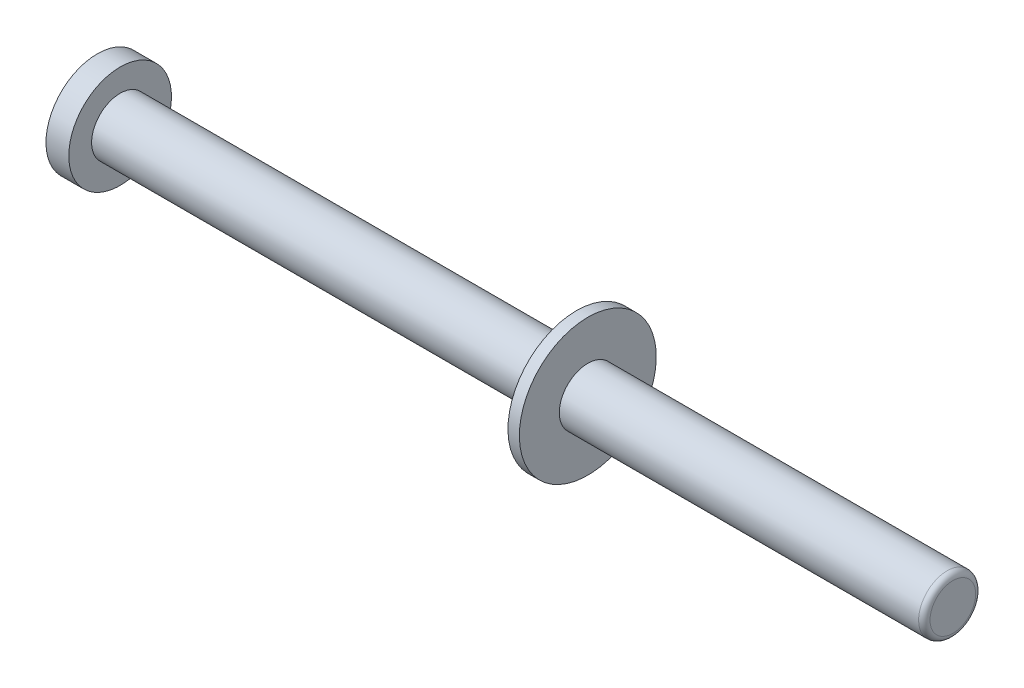
ISO-10303-21;
HEADER;
FILE_DESCRIPTION(('STEP AP214'),'2;1');
FILE_NAME('part.step','',(''),(''),'','','');
FILE_SCHEMA(('AUTOMOTIVE_DESIGN { 1 0 10303 214 1 1 1 1 }'));
ENDSEC;
DATA;
#1=APPLICATION_CONTEXT('core data for automotive mechanical design processes');
#2=APPLICATION_PROTOCOL_DEFINITION('international standard','automotive_design',2000,#1);
#3=PRODUCT_CONTEXT('',#1,'mechanical');
#4=PRODUCT('Part','Part','',(#3));
#5=PRODUCT_RELATED_PRODUCT_CATEGORY('part','',(#4));
#6=PRODUCT_DEFINITION_FORMATION('','',#4);
#7=PRODUCT_DEFINITION_CONTEXT('part definition',#1,'design');
#8=PRODUCT_DEFINITION('design','',#6,#7);
#9=PRODUCT_DEFINITION_SHAPE('','',#8);
#10=(LENGTH_UNIT() NAMED_UNIT(*) SI_UNIT(.MILLI.,.METRE.));
#11=(NAMED_UNIT(*) PLANE_ANGLE_UNIT() SI_UNIT($,.RADIAN.));
#12=(NAMED_UNIT(*) SI_UNIT($,.STERADIAN.) SOLID_ANGLE_UNIT());
#13=UNCERTAINTY_MEASURE_WITH_UNIT(LENGTH_MEASURE(1.E-05),#10,'distance_accuracy_value','');
#14=(GEOMETRIC_REPRESENTATION_CONTEXT(3) GLOBAL_UNCERTAINTY_ASSIGNED_CONTEXT((#13)) GLOBAL_UNIT_ASSIGNED_CONTEXT((#10,
#11,#12)) REPRESENTATION_CONTEXT('',''));
#15=CARTESIAN_POINT('',(0.,0.,0.));
#16=DIRECTION('',(0.,0.,1.));
#17=DIRECTION('',(1.,0.,0.));
#18=AXIS2_PLACEMENT_3D('',#15,#16,#17);
#19=CARTESIAN_POINT('',(-150.,0.,0.));
#20=DIRECTION('',(-1.,0.,0.));
#21=DIRECTION('',(0.,-1.,0.));
#22=AXIS2_PLACEMENT_3D('',#19,#20,#21);
#23=PLANE('',#22);
#24=CARTESIAN_POINT('',(-150.,0.,0.));
#25=DIRECTION('',(1.,0.,0.));
#26=DIRECTION('',(0.,1.,0.));
#27=AXIS2_PLACEMENT_3D('',#24,#25,#26);
#28=CIRCLE('',#27,9.00000000000001);
#29=CARTESIAN_POINT('',(-150.,9.,0.));
#30=VERTEX_POINT('',#29);
#31=EDGE_CURVE('E49',#30,#30,#28,.T.);
#32=ORIENTED_EDGE('',*,*,#31,.F.);
#33=EDGE_LOOP('',(#32));
#34=FACE_BOUND('',#33,.T.);
#35=ADVANCED_FACE('F39',(#34),#23,.T.);
#36=CARTESIAN_POINT('',(0.,0.,0.));
#37=DIRECTION('',(1.,0.,0.));
#38=DIRECTION('',(0.,1.,0.));
#39=AXIS2_PLACEMENT_3D('',#36,#37,#38);
#40=CYLINDRICAL_SURFACE('',#39,9.00000000000001);
#41=ORIENTED_EDGE('',*,*,#31,.T.);
#42=EDGE_LOOP('',(#41));
#43=FACE_BOUND('',#42,.T.);
#44=CARTESIAN_POINT('',(-146.,0.,0.));
#45=DIRECTION('',(1.,0.,0.));
#46=DIRECTION('',(0.,1.,0.));
#47=AXIS2_PLACEMENT_3D('',#44,#45,#46);
#48=CIRCLE('',#47,9.00000000000001);
#49=CARTESIAN_POINT('',(-146.,9.,0.));
#50=VERTEX_POINT('',#49);
#51=EDGE_CURVE('E53',#50,#50,#48,.T.);
#52=ORIENTED_EDGE('',*,*,#51,.F.);
#53=EDGE_LOOP('',(#52));
#54=FACE_BOUND('',#53,.T.);
#55=ADVANCED_FACE('F95',(#43,#54),#40,.T.);
#56=CARTESIAN_POINT('',(-146.,9.,0.));
#57=DIRECTION('',(1.,0.,0.));
#58=DIRECTION('',(0.,1.,0.));
#59=AXIS2_PLACEMENT_3D('',#56,#57,#58);
#60=PLANE('',#59);
#61=ORIENTED_EDGE('',*,*,#51,.T.);
#62=EDGE_LOOP('',(#61));
#63=FACE_BOUND('',#62,.T.);
#64=CARTESIAN_POINT('',(-146.,0.,0.));
#65=DIRECTION('',(1.,0.,0.));
#66=DIRECTION('',(0.,1.,0.));
#67=AXIS2_PLACEMENT_3D('',#64,#65,#66);
#68=CIRCLE('',#67,5.00000000000001);
#69=CARTESIAN_POINT('',(-146.,5.,0.));
#70=VERTEX_POINT('',#69);
#71=EDGE_CURVE('E56',#70,#70,#68,.T.);
#72=ORIENTED_EDGE('',*,*,#71,.F.);
#73=EDGE_LOOP('',(#72));
#74=FACE_BOUND('',#73,.T.);
#75=ADVANCED_FACE('F100',(#63,#74),#60,.T.);
#76=CARTESIAN_POINT('',(0.,0.,0.));
#77=DIRECTION('',(1.,0.,0.));
#78=DIRECTION('',(0.,1.,0.));
#79=AXIS2_PLACEMENT_3D('',#76,#77,#78);
#80=CYLINDRICAL_SURFACE('',#79,5.00000000000001);
#81=ORIENTED_EDGE('',*,*,#71,.T.);
#82=EDGE_LOOP('',(#81));
#83=FACE_BOUND('',#82,.T.);
#84=CARTESIAN_POINT('',(-66.,0.,0.));
#85=DIRECTION('',(1.,0.,0.));
#86=DIRECTION('',(0.,1.,0.));
#87=AXIS2_PLACEMENT_3D('',#84,#85,#86);
#88=CIRCLE('',#87,5.00000000000001);
#89=CARTESIAN_POINT('',(-66.,5.,0.));
#90=VERTEX_POINT('',#89);
#91=EDGE_CURVE('E61',#90,#90,#88,.T.);
#92=ORIENTED_EDGE('',*,*,#91,.F.);
#93=EDGE_LOOP('',(#92));
#94=FACE_BOUND('',#93,.T.);
#95=ADVANCED_FACE('F102',(#83,#94),#80,.T.);
#96=CARTESIAN_POINT('',(-66.,5.,0.));
#97=DIRECTION('',(-1.,0.,0.));
#98=DIRECTION('',(0.,-1.,0.));
#99=AXIS2_PLACEMENT_3D('',#96,#97,#98);
#100=PLANE('',#99);
#101=ORIENTED_EDGE('',*,*,#91,.T.);
#102=EDGE_LOOP('',(#101));
#103=FACE_BOUND('',#102,.T.);
#104=CARTESIAN_POINT('',(-66.,0.,0.));
#105=DIRECTION('',(1.,0.,0.));
#106=DIRECTION('',(0.,1.,0.));
#107=AXIS2_PLACEMENT_3D('',#104,#105,#106);
#108=CIRCLE('',#107,12.);
#109=CARTESIAN_POINT('',(-66.,12.,0.));
#110=VERTEX_POINT('',#109);
#111=EDGE_CURVE('E62',#110,#110,#108,.T.);
#112=ORIENTED_EDGE('',*,*,#111,.F.);
#113=EDGE_LOOP('',(#112));
#114=FACE_BOUND('',#113,.T.);
#115=ADVANCED_FACE('F86',(#103,#114),#100,.T.);
#116=CARTESIAN_POINT('',(0.,0.,0.));
#117=DIRECTION('',(1.,0.,0.));
#118=DIRECTION('',(0.,1.,0.));
#119=AXIS2_PLACEMENT_3D('',#116,#117,#118);
#120=CYLINDRICAL_SURFACE('',#119,12.);
#121=ORIENTED_EDGE('',*,*,#111,.T.);
#122=EDGE_LOOP('',(#121));
#123=FACE_BOUND('',#122,.T.);
#124=CARTESIAN_POINT('',(-64.,0.,0.));
#125=DIRECTION('',(1.,0.,0.));
#126=DIRECTION('',(0.,1.,0.));
#127=AXIS2_PLACEMENT_3D('',#124,#125,#126);
#128=CIRCLE('',#127,12.);
#129=CARTESIAN_POINT('',(-64.,12.,0.));
#130=VERTEX_POINT('',#129);
#131=EDGE_CURVE('E68',#130,#130,#128,.T.);
#132=ORIENTED_EDGE('',*,*,#131,.F.);
#133=EDGE_LOOP('',(#132));
#134=FACE_BOUND('',#133,.T.);
#135=ADVANCED_FACE('F78',(#123,#134),#120,.T.);
#136=CARTESIAN_POINT('',(-64.,12.,0.));
#137=DIRECTION('',(1.,0.,0.));
#138=DIRECTION('',(0.,1.,0.));
#139=AXIS2_PLACEMENT_3D('',#136,#137,#138);
#140=PLANE('',#139);
#141=ORIENTED_EDGE('',*,*,#131,.T.);
#142=EDGE_LOOP('',(#141));
#143=FACE_BOUND('',#142,.T.);
#144=CARTESIAN_POINT('',(-64.,0.,0.));
#145=DIRECTION('',(1.,0.,0.));
#146=DIRECTION('',(0.,1.,0.));
#147=AXIS2_PLACEMENT_3D('',#144,#145,#146);
#148=CIRCLE('',#147,5.00000000000001);
#149=CARTESIAN_POINT('',(-64.,5.,0.));
#150=VERTEX_POINT('',#149);
#151=EDGE_CURVE('E72',#150,#150,#148,.T.);
#152=ORIENTED_EDGE('',*,*,#151,.F.);
#153=EDGE_LOOP('',(#152));
#154=FACE_BOUND('',#153,.T.);
#155=ADVANCED_FACE('F76',(#143,#154),#140,.T.);
#156=CARTESIAN_POINT('',(0.,0.,0.));
#157=DIRECTION('',(1.,0.,0.));
#158=DIRECTION('',(0.,1.,0.));
#159=AXIS2_PLACEMENT_3D('',#156,#157,#158);
#160=CYLINDRICAL_SURFACE('',#159,5.);
#161=CARTESIAN_POINT('',(-1.,0.,0.));
#162=DIRECTION('',(1.,0.,0.));
#163=DIRECTION('',(0.,1.,0.));
#164=AXIS2_PLACEMENT_3D('',#161,#162,#163);
#165=CIRCLE('',#164,5.);
#166=CARTESIAN_POINT('',(-1.,5.,0.));
#167=VERTEX_POINT('',#166);
#168=EDGE_CURVE('E10',#167,#167,#165,.F.);
#169=ORIENTED_EDGE('',*,*,#168,.T.);
#170=EDGE_LOOP('',(#169));
#171=FACE_BOUND('',#170,.T.);
#172=ORIENTED_EDGE('',*,*,#151,.T.);
#173=EDGE_LOOP('',(#172));
#174=FACE_BOUND('',#173,.T.);
#175=ADVANCED_FACE('F73',(#171,#174),#160,.T.);
#176=CARTESIAN_POINT('',(0.,5.,0.));
#177=DIRECTION('',(1.,0.,0.));
#178=DIRECTION('',(0.,1.,0.));
#179=AXIS2_PLACEMENT_3D('',#176,#177,#178);
#180=PLANE('',#179);
#181=CARTESIAN_POINT('',(0.,0.,0.));
#182=DIRECTION('',(1.,0.,0.));
#183=DIRECTION('',(0.,1.,0.));
#184=AXIS2_PLACEMENT_3D('',#181,#182,#183);
#185=CIRCLE('',#184,4.);
#186=CARTESIAN_POINT('',(0.,4.,0.));
#187=VERTEX_POINT('',#186);
#188=EDGE_CURVE('E46',#187,#187,#185,.T.);
#189=ORIENTED_EDGE('',*,*,#188,.T.);
#190=EDGE_LOOP('',(#189));
#191=FACE_BOUND('',#190,.T.);
#192=ADVANCED_FACE('F88',(#191),#180,.T.);
#193=CARTESIAN_POINT('',(-1.,0.,0.));
#194=DIRECTION('',(1.,0.,0.));
#195=DIRECTION('',(0.,1.,0.));
#196=AXIS2_PLACEMENT_3D('',#193,#194,#195);
#197=TOROIDAL_SURFACE('',#196,4.,1.);
#198=ORIENTED_EDGE('',*,*,#168,.F.);
#199=EDGE_LOOP('',(#198));
#200=FACE_BOUND('',#199,.T.);
#201=ORIENTED_EDGE('',*,*,#188,.F.);
#202=EDGE_LOOP('',(#201));
#203=FACE_BOUND('',#202,.T.);
#204=ADVANCED_FACE('F41',(#200,#203),#197,.T.);
#205=CLOSED_SHELL('',(#35,#55,#75,#95,#115,#135,#155,#175,#192,#204));
#206=MANIFOLD_SOLID_BREP('B2',#205);
#207=ADVANCED_BREP_SHAPE_REPRESENTATION('',(#18,#206),#14);
#208=SHAPE_DEFINITION_REPRESENTATION(#9,#207);
ENDSEC;
END-ISO-10303-21;
